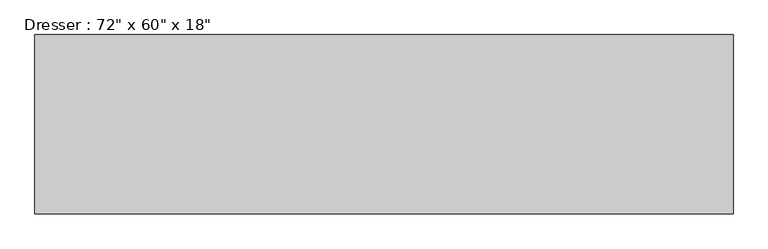
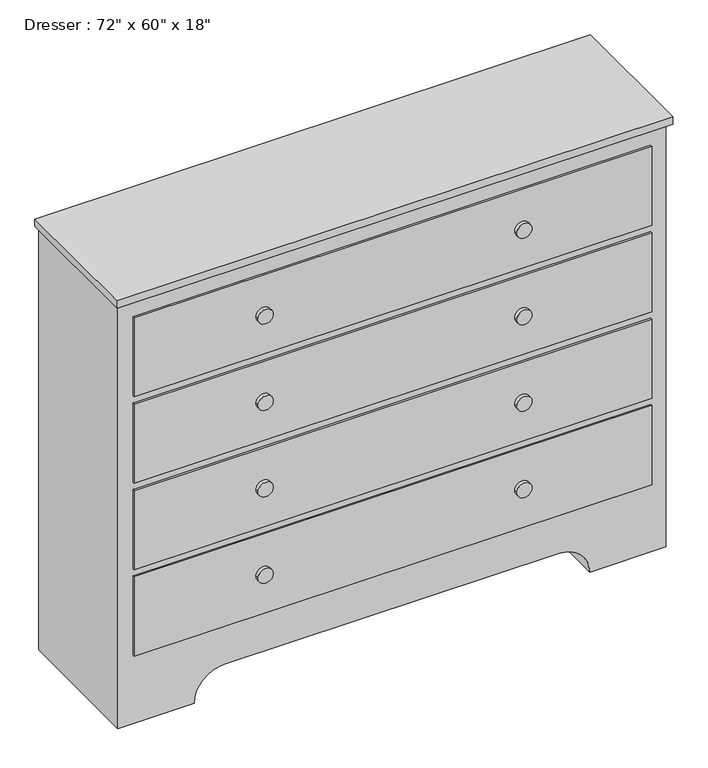
"""IFC4 building model written with IfcOpenShell, lengths in millimetres: furniture geometry."""

from ifc_helpers import new_model, si_unit, point, frame, frame_2d, origin, place, context, project, spatial, polyline, circle_curve, trimmed, segment, composite_curve, outline, extrude, source, transform, mapped, element, save


def furniture_7c473f12(model_context):
    return source(origin(), model_context, "Body", "SweptSolid", [
        extrude(outline(polyline([(657.9067402, -134.5629541), (657.9067402, -610.8129541), (-1196.2932598, -610.8129541), (-1196.2932598, -134.5629541), (657.9067402, -134.5629541)])), frame((0.0, 0.0, 1498.6), z_axis=(0.0, 0.0, 1.0), x_axis=(1.0, 0.0, 0.0)), (0.0, 0.0, 1.0), 25.4),
        extrude(outline(composite_curve([segment(polyline([(0.0, 645.2067402), (1498.6, 645.2067402), (1498.6, -1183.5932598), (0.0, -1183.5932598), (0.0, -929.5932598)]), True, "CONTINUOUS"), segment(trimmed(circle_curve(frame_2d((0.0, -827.9932598)), 101.6), [point((0.0, -929.5932598))], [point((101.6, -827.9932598))], True, "CARTESIAN"), True, "CONTINUOUS"), segment(polyline([(101.6, -827.9932598), (101.6, 289.6067402)]), True, "CONTINUOUS"), segment(trimmed(circle_curve(frame_2d((0.0, 289.6067402)), 101.6), [point((101.6, 289.6067402))], [point((0.0, 391.2067402))], True, "CARTESIAN"), True, "CONTINUOUS"), segment(polyline([(0.0, 391.2067402), (0.0, 645.2067402)]), True, "CONTINUOUS")], self_intersect=False)), frame((0.0, -591.7629541, 0.0), z_axis=(0.0, 1.0, 0.0), x_axis=(0.0, 0.0, 1.0)), (0.0, 0.0, 1.0), 457.2),
        extrude(outline(composite_curve([segment(trimmed(circle_curve(frame_2d((1295.4, 162.6067402)), 25.4), [point((1295.4, 137.2067402))], [point((1295.4, 188.0067402))], False, "CARTESIAN"), True, "CONTINUOUS"), segment(trimmed(circle_curve(frame_2d((1295.4, 162.6067402)), 25.4), [point((1295.4, 188.0067402))], [point((1295.4, 137.2067402))], False, "CARTESIAN"), True, "CONTINUOUS")], self_intersect=False)), frame((0.0, -610.8129541, 0.0), z_axis=(0.0, 1.0, 0.0), x_axis=(0.0, 0.0, 1.0)), (0.0, 0.0, 1.0), 12.7),
        extrude(outline(composite_curve([segment(trimmed(circle_curve(frame_2d((990.6, 162.6067402)), 25.4), [point((990.6, 137.2067402))], [point((990.6, 188.0067402))], False, "CARTESIAN"), True, "CONTINUOUS"), segment(trimmed(circle_curve(frame_2d((990.6, 162.6067402)), 25.4), [point((990.6, 188.0067402))], [point((990.6, 137.2067402))], False, "CARTESIAN"), True, "CONTINUOUS")], self_intersect=False)), frame((0.0, -610.8129541, 0.0), z_axis=(0.0, 1.0, 0.0), x_axis=(0.0, 0.0, 1.0)), (0.0, 0.0, 1.0), 12.7),
        extrude(outline(composite_curve([segment(trimmed(circle_curve(frame_2d((685.8, 162.6067402)), 25.4), [point((685.8, 137.2067402))], [point((685.8, 188.0067402))], False, "CARTESIAN"), True, "CONTINUOUS"), segment(trimmed(circle_curve(frame_2d((685.8, 162.6067402)), 25.4), [point((685.8, 188.0067402))], [point((685.8, 137.2067402))], False, "CARTESIAN"), True, "CONTINUOUS")], self_intersect=False)), frame((0.0, -610.8129541, 0.0), z_axis=(0.0, 1.0, 0.0), x_axis=(0.0, 0.0, 1.0)), (0.0, 0.0, 1.0), 12.7),
        extrude(outline(composite_curve([segment(trimmed(circle_curve(frame_2d((381.0, 162.6067402)), 25.4), [point((381.0, 137.2067402))], [point((381.0, 188.0067402))], False, "CARTESIAN"), True, "CONTINUOUS"), segment(trimmed(circle_curve(frame_2d((381.0, 162.6067402)), 25.4), [point((381.0, 188.0067402))], [point((381.0, 137.2067402))], False, "CARTESIAN"), True, "CONTINUOUS")], self_intersect=False)), frame((0.0, -610.8129541, 0.0), z_axis=(0.0, 1.0, 0.0), x_axis=(0.0, 0.0, 1.0)), (0.0, 0.0, 1.0), 12.7),
        extrude(outline(composite_curve([segment(trimmed(circle_curve(frame_2d((381.0, -700.9932598)), 25.4), [point((381.0, -726.3932598))], [point((381.0, -675.5932598))], False, "CARTESIAN"), True, "CONTINUOUS"), segment(trimmed(circle_curve(frame_2d((381.0, -700.9932598)), 25.4), [point((381.0, -675.5932598))], [point((381.0, -726.3932598))], False, "CARTESIAN"), True, "CONTINUOUS")], self_intersect=False)), frame((0.0, -610.8129541, 0.0), z_axis=(0.0, 1.0, 0.0), x_axis=(0.0, 0.0, 1.0)), (0.0, 0.0, 1.0), 12.7),
        extrude(outline(composite_curve([segment(trimmed(circle_curve(frame_2d((685.8, -700.9932598)), 25.4), [point((685.8, -726.3932598))], [point((685.8, -675.5932598))], False, "CARTESIAN"), True, "CONTINUOUS"), segment(trimmed(circle_curve(frame_2d((685.8, -700.9932598)), 25.4), [point((685.8, -675.5932598))], [point((685.8, -726.3932598))], False, "CARTESIAN"), True, "CONTINUOUS")], self_intersect=False)), frame((0.0, -610.8129541, 0.0), z_axis=(0.0, 1.0, 0.0), x_axis=(0.0, 0.0, 1.0)), (0.0, 0.0, 1.0), 12.7),
        extrude(outline(composite_curve([segment(trimmed(circle_curve(frame_2d((990.6, -700.9932598)), 25.4), [point((990.6, -726.3932598))], [point((990.6, -675.5932598))], False, "CARTESIAN"), True, "CONTINUOUS"), segment(trimmed(circle_curve(frame_2d((990.6, -700.9932598)), 25.4), [point((990.6, -675.5932598))], [point((990.6, -726.3932598))], False, "CARTESIAN"), True, "CONTINUOUS")], self_intersect=False)), frame((0.0, -610.8129541, 0.0), z_axis=(0.0, 1.0, 0.0), x_axis=(0.0, 0.0, 1.0)), (0.0, 0.0, 1.0), 12.7),
        extrude(outline(composite_curve([segment(trimmed(circle_curve(frame_2d((1295.4, -700.9932598)), 25.4), [point((1295.4, -726.3932598))], [point((1295.4, -675.5932598))], False, "CARTESIAN"), True, "CONTINUOUS"), segment(trimmed(circle_curve(frame_2d((1295.4, -700.9932598)), 25.4), [point((1295.4, -675.5932598))], [point((1295.4, -726.3932598))], False, "CARTESIAN"), True, "CONTINUOUS")], self_intersect=False)), frame((0.0, -610.8129541, 0.0), z_axis=(0.0, 1.0, 0.0), x_axis=(0.0, 0.0, 1.0)), (0.0, 0.0, 1.0), 12.7),
        extrude(outline(polyline([(594.4067402, -598.1129541), (-1132.7932598, -598.1129541), (-1132.7932598, -591.7629541), (594.4067402, -591.7629541), (594.4067402, -598.1129541)])), frame((0.0, 0.0, 1155.7), z_axis=(0.0, 0.0, 1.0), x_axis=(1.0, 0.0, 0.0)), (0.0, 0.0, 1.0), 279.4),
        extrude(outline(polyline([(594.4067402, -598.1129541), (-1132.7932598, -598.1129541), (-1132.7932598, -591.7629541), (594.4067402, -591.7629541), (594.4067402, -598.1129541)])), frame((0.0, 0.0, 850.9), z_axis=(0.0, 0.0, 1.0), x_axis=(1.0, 0.0, 0.0)), (0.0, 0.0, 1.0), 279.4),
        extrude(outline(polyline([(594.4067402, -598.1129541), (-1132.7932598, -598.1129541), (-1132.7932598, -591.7629541), (594.4067402, -591.7629541), (594.4067402, -598.1129541)])), frame((0.0, 0.0, 546.1), z_axis=(0.0, 0.0, 1.0), x_axis=(1.0, 0.0, 0.0)), (0.0, 0.0, 1.0), 279.4),
        extrude(outline(polyline([(594.4067402, -598.1129541), (-1132.7932598, -598.1129541), (-1132.7932598, -591.7629541), (594.4067402, -591.7629541), (594.4067402, -598.1129541)])), frame((0.0, 0.0, 241.3), z_axis=(0.0, 0.0, 1.0), x_axis=(1.0, 0.0, 0.0)), (0.0, 0.0, 1.0), 279.4),
    ])


if __name__ == "__main__":
    model = new_model("IFC4")
    model_context = context("Model", 3, world=origin())
    ifc_project = project(units=[si_unit("LENGTHUNIT", "METRE", prefix="MILLI")], contexts=[model_context])
    site = spatial("IfcSite", under=ifc_project)
    building = spatial("IfcBuilding", under=site)
    placement = place(None, origin())
    furniture_shape = furniture_7c473f12(model_context)
    element("IfcFurniture", 1, ObjectType="Dresser : 72\" x 60\" x 18\"", at=placement, inside=building, context=model_context, shape_type="MappedRepresentation", body=[
        mapped(furniture_shape, transform((0.0, 0.0, 0.0), x_axis=(1.0, 0.0, 0.0), y_axis=(0.0, 1.0, 0.0), z_axis=(0.0, 0.0, 1.0))),
    ])
    save(model, "model.ifc")

# Revit data of these elements
# Type "Dresser : 72\" x 60\" x 18\""
#   Assembly Code = "E2020200"
#   Depth = 1' - 6"
#   Height = 5' - 0"
#   Width = 6' - 0"
#   Dresser Material = Laminate - Ivory, Glossy
#   Drawer Material = Laminate, Ivory, Matte
#   Knob Material = Cherry
#   Default Elevation = 0
# Element 1 (IfcFurniture, "Dresser : 72\" x 60\" x 18\"")
#   Materials on its faces: "Laminate, Ivory, Matte", "Cherry", "Laminate - Ivory, Glossy"
# Materials
#   "Laminate - Ivory, Glossy": colour RGB 247 247 239, transparency 0
#   "Laminate, Ivory, Matte": class "Plastic", colour RGB 247 247 239, transparency 0, Description = "Plastic Laminate - Ivory, Matte", Cost = 0
#   "Cherry": class "Wood", colour RGB 226 177 128, transparency 0, Description = "Prunus Serotina", Cost = 0
